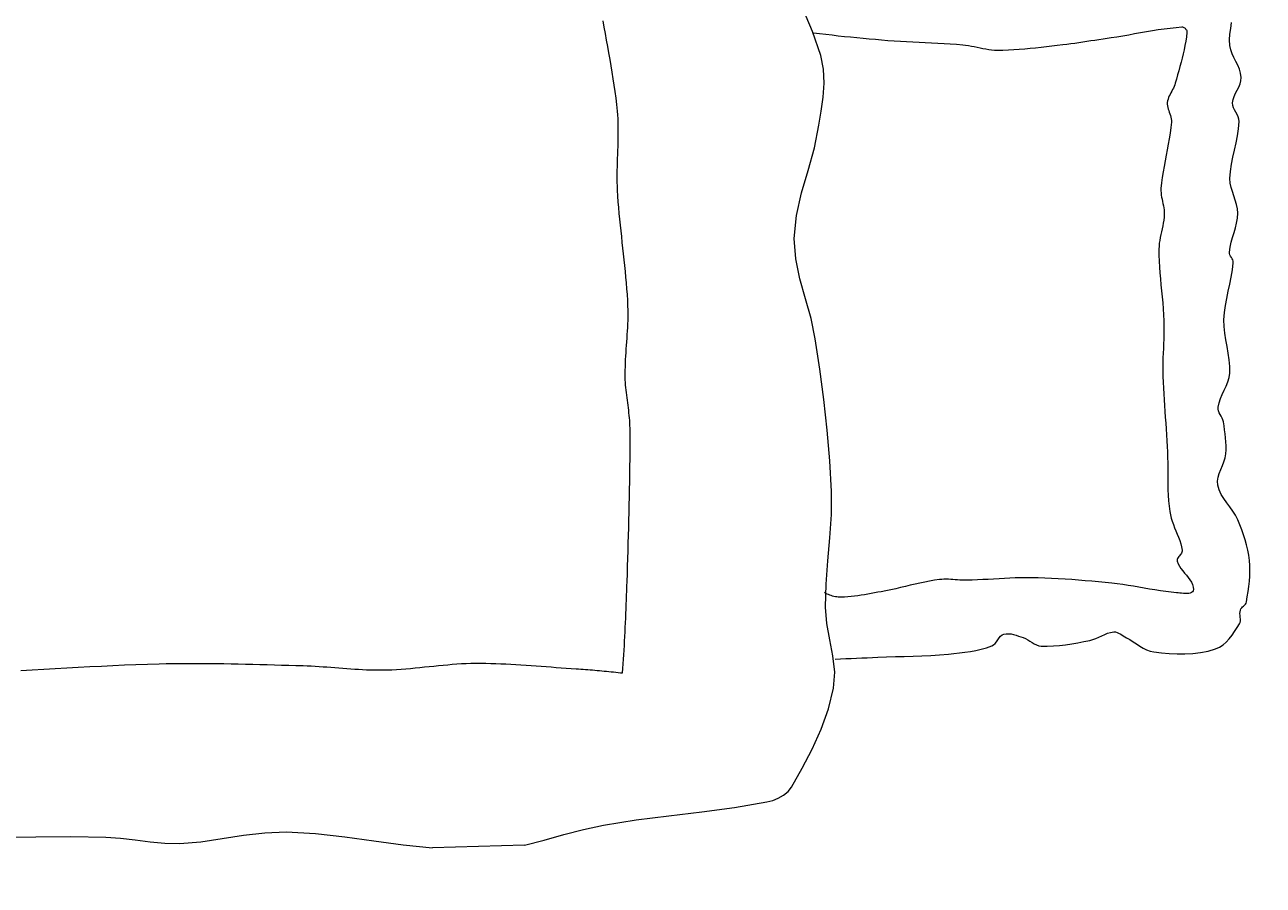
# Model space of a CAD drawing. Units: inches. Extents: x 1441 to 2460, y 1648 to 2683.
# Tile 5 of 35: x 1830 to 1880, y 1866 to 1901. Entities that reach past the tile are written whole.
import ezdxf

# ---------------------------------------------------------------- set-up
doc = ezdxf.new("R2010")
doc.units = ezdxf.units.IN
doc.layers.add('A-ANNO-DIMS', color=2, linetype='Continuous', lineweight=18)
doc.layers.add('A-FURN', color=8, linetype='Continuous', lineweight=15)
doc.styles.get("Standard").update_dxf_attribs({"font": 'arial.ttf'})
doc.dimstyles.get("Standard").update_dxf_attribs({"dimtxt": 0.18, "dimasz": 0.18, "dimexe": 0.18, "dimexo": 0.0625, "dimgap": 0.09, "dimtad": 0, "dimtih": 1, "dimtoh": 1, "dimdec": 4, "dimzin": 0, "dimdsep": 46, "dimtxsty": 'Standard', "dimcen": 0.09, "dimadec": 0, "dimazin": 0, "dimtfac": 1, "dimtdec": 4, "dimtofl": 0, "dimtmove": 0, "dimatfit": 3, "dimfxl": 1, "dimtolj": 1, "dimtzin": 0, "dimarcsym": 0})

# ---------------------------------------------------------------- blocks, each defined once
blk = doc.blocks.new('BED-DOUBLE-PLAN')
for p, q in [((52.61, 91.603), (52.404, 91.554)), ((52.818, 91.642), (52.61, 91.603)), ((53.027, 91.67), (52.818, 91.642)), ((53.234, 91.686), (53.027, 91.67)), ((53.441, 91.69), (53.234, 91.686)), ((53.649, 91.684), (53.441, 91.69)), ((53.857, 91.67), (53.649, 91.684)), ((54.065, 91.648), (53.857, 91.67)), ((54.272, 91.619), (54.065, 91.648)), ((54.478, 91.587), (54.272, 91.619)), ((54.683, 91.551), (54.478, 91.587)), ((33.099, 91.129), (32.945, 91.051)), ((33.253, 91.205), (33.099, 91.129)), ((33.41, 91.271), (33.253, 91.205)), ((33.569, 91.32), (33.41, 91.271)), ((33.735, 91.343), (33.569, 91.32)), ((33.867, 91.333), (33.735, 91.343)), ((33.995, 91.298), (33.867, 91.333)), ((34.121, 91.245), (33.995, 91.298)), ((34.245, 91.181), (34.121, 91.245)), ((34.37, 91.117), (34.245, 91.181)), ((34.495, 91.058), (34.37, 91.117)), ((35.036, 91.076), (34.945, 91.032)), ((35.126, 91.127), (35.036, 91.076)), ((35.216, 91.178), (35.126, 91.127)), ((35.307, 91.222), (35.216, 91.178)), ((35.4, 91.252), (35.307, 91.222)), ((35.496, 91.261), (35.4, 91.252)), ((35.784, 91.238), (35.496, 91.261)), ((36.07, 91.194), (35.784, 91.238)), ((36.354, 91.135), (36.07, 91.194)), ((36.638, 91.07), (36.354, 91.135)), ((36.922, 91.006), (36.638, 91.07)), ((38.639, 91.107), (38.469, 91.048)), ((38.81, 91.159), (38.639, 91.107)), ((38.983, 91.195), (38.81, 91.159)), ((39.158, 91.208), (38.983, 91.195)), ((39.356, 91.195), (39.158, 91.208)), ((39.551, 91.161), (39.356, 91.195)), ((39.744, 91.114), (39.551, 91.161)), ((39.936, 91.058), (39.744, 91.114)), ((51.224, 91.115), (51.053, 91.006)), ((51.403, 91.204), (51.224, 91.115)), ((51.599, 91.285), (51.403, 91.204)), ((51.797, 91.361), (51.599, 91.285)), ((51.997, 91.432), (51.797, 91.361)), ((52.2, 91.497), (51.997, 91.432)), ((52.404, 91.554), (52.2, 91.497)), ((54.729, 91.535), (54.683, 91.551)), ((54.771, 91.509), (54.729, 91.535)), ((54.81, 91.475), (54.771, 91.509)), ((54.847, 91.437), (54.81, 91.475)), ((54.884, 91.398), (54.847, 91.437)), ((54.922, 91.361), (54.884, 91.398)), ((54.963, 91.331), (54.922, 91.361)), ((55.008, 91.31), (54.963, 91.331)), ((55.076, 91.296), (55.008, 91.31)), ((55.147, 91.294), (55.076, 91.296)), ((55.219, 91.299), (55.147, 91.294)), ((55.292, 91.306), (55.219, 91.299)), ((55.364, 91.311), (55.292, 91.306)), ((55.433, 91.31), (55.364, 91.311)), ((55.499, 91.298), (55.433, 91.31)), ((55.56, 91.27), (55.499, 91.298)), ((55.709, 91.176), (55.56, 91.27)), ((55.86, 91.078), (55.709, 91.176)), ((56.01, 90.975), (55.86, 91.078)), ((31.78, 90.922), (31.549, 90.959)), ((32.011, 90.889), (31.78, 90.922)), ((32.24, 90.873), (32.011, 90.889)), ((32.466, 90.885), (32.24, 90.873)), ((32.63, 90.922), (32.466, 90.885)), ((32.789, 90.98), (32.63, 90.922)), ((32.945, 91.051), (32.789, 90.98)), ((34.624, 91.015), (34.495, 91.058)), ((34.756, 90.994), (34.624, 91.015)), ((34.852, 91.003), (34.756, 90.994)), ((34.945, 91.032), (34.852, 91.003)), ((37.206, 90.949), (36.922, 91.006)), ((37.492, 90.908), (37.206, 90.949)), ((37.78, 90.89), (37.492, 90.908)), ((37.955, 90.902), (37.78, 90.89)), ((38.128, 90.938), (37.955, 90.902)), ((38.299, 90.989), (38.128, 90.938)), ((38.469, 91.048), (38.299, 90.989)), ((40.129, 91), (39.936, 91.058)), ((40.322, 90.946), (40.129, 91)), ((40.516, 90.901), (40.322, 90.946)), ((40.713, 90.873), (40.516, 90.901)), ((40.767, 90.876), (40.713, 90.873)), ((40.821, 90.893), (40.767, 90.876)), ((40.873, 90.918), (40.821, 90.893)), ((40.924, 90.949), (40.873, 90.918)), ((40.975, 90.979), (40.924, 90.949)), ((41.027, 91.005), (40.975, 90.979)), ((41.081, 91.022), (41.027, 91.005)), ((41.135, 91.025), (41.081, 91.022)), ((41.423, 90.993), (41.135, 91.025)), ((41.708, 90.945), (41.423, 90.993)), ((41.993, 90.887), (41.708, 90.945)), ((42.277, 90.826), (41.993, 90.887)), ((42.561, 90.766), (42.277, 90.826)), ((42.845, 90.714), (42.561, 90.766)), ((43.131, 90.675), (42.845, 90.714)), ((43.419, 90.654), (43.131, 90.675)), ((43.686, 90.66), (43.419, 90.654)), ((43.952, 90.687), (43.686, 90.66)), ((44.218, 90.73), (43.952, 90.687)), ((44.483, 90.779), (44.218, 90.73)), ((44.748, 90.826), (44.483, 90.779)), ((45.014, 90.865), (44.748, 90.826)), ((45.28, 90.887), (45.014, 90.865)), ((45.546, 90.884), (45.28, 90.887)), ((45.723, 90.857), (45.546, 90.884)), ((45.894, 90.807), (45.723, 90.857)), ((46.062, 90.739), (45.894, 90.807)), ((46.228, 90.663), (46.062, 90.739)), ((46.394, 90.585), (46.228, 90.663)), ((46.562, 90.514), (46.394, 90.585)), ((47.342, 90.578), (47.27, 90.541)), ((47.415, 90.609), (47.342, 90.578)), ((47.49, 90.629), (47.415, 90.609)), ((47.648, 90.655), (47.49, 90.629)), ((47.807, 90.68), (47.648, 90.655)), ((47.967, 90.702), (47.807, 90.68)), ((48.127, 90.721), (47.967, 90.702)), ((48.287, 90.734), (48.127, 90.721)), ((48.447, 90.741), (48.287, 90.734)), ((48.607, 90.741), (48.447, 90.741)), ((48.767, 90.731), (48.607, 90.741)), ((48.926, 90.703), (48.767, 90.731)), ((49.084, 90.654), (48.926, 90.703)), ((49.24, 90.592), (49.084, 90.654)), ((49.395, 90.526), (49.24, 90.592)), ((50.558, 90.646), (50.387, 90.542)), ((50.723, 90.763), (50.558, 90.646)), ((50.888, 90.886), (50.723, 90.763)), ((51.053, 91.006), (50.888, 90.886)), ((56.153, 90.865), (56.01, 90.975)), ((56.284, 90.746), (56.153, 90.865)), ((56.399, 90.616), (56.284, 90.746)), ((56.493, 90.473), (56.399, 90.616)), ((46.733, 90.456), (46.562, 90.514)), ((46.908, 90.42), (46.733, 90.456)), ((46.984, 90.419), (46.908, 90.42)), ((47.057, 90.436), (46.984, 90.419)), ((47.128, 90.465), (47.057, 90.436)), ((47.199, 90.502), (47.128, 90.465)), ((47.27, 90.541), (47.199, 90.502)), ((49.549, 90.466), (49.395, 90.526)), ((49.704, 90.42), (49.549, 90.466)), ((49.861, 90.397), (49.704, 90.42)), ((50.019, 90.406), (49.861, 90.397)), ((50.209, 90.459), (50.019, 90.406)), ((50.387, 90.542), (50.209, 90.459)), ((56.561, 90.317), (56.493, 90.473)), ((56.643, 90.02), (56.561, 90.317)), ((56.701, 89.716), (56.643, 90.02)), ((56.736, 89.408), (56.701, 89.716)), ((31.755, 89.074), (31.774, 89.097)), ((31.774, 89.097), (31.795, 89.117)), ((31.795, 89.117), (31.818, 89.136)), ((31.818, 89.136), (31.843, 89.151)), ((31.843, 89.151), (31.869, 89.163)), ((31.869, 89.163), (31.896, 89.172)), ((31.896, 89.172), (31.922, 89.176)), ((31.922, 89.176), (31.948, 89.176)), ((31.948, 89.176), (32.119, 89.153)), ((32.119, 89.153), (32.29, 89.126)), ((32.29, 89.126), (32.459, 89.095)), ((32.459, 89.095), (32.629, 89.06)), ((53.527, 89.081), (53.616, 89.156)), ((53.616, 89.156), (53.705, 89.228)), ((53.705, 89.228), (53.796, 89.294)), ((53.796, 89.294), (53.889, 89.351)), ((53.889, 89.351), (53.985, 89.396)), ((53.985, 89.396), (54.086, 89.424)), ((54.086, 89.424), (54.192, 89.433)), ((54.192, 89.433), (54.243, 89.423)), ((54.243, 89.423), (54.282, 89.397)), ((54.282, 89.397), (54.31, 89.358)), ((54.31, 89.358), (54.329, 89.307)), ((54.329, 89.307), (54.341, 89.247)), ((54.341, 89.247), (54.346, 89.18)), ((54.346, 89.109), (54.342, 89.035)), ((54.346, 89.18), (54.346, 89.109)), ((56.752, 89.096), (56.736, 89.408)), ((56.751, 88.783), (56.752, 89.096)), ((31.722, 88.975), (31.723, 89)), ((31.741, 88.737), (31.722, 88.975)), ((31.723, 89), (31.729, 89.025)), ((31.729, 89.025), (31.74, 89.05)), ((31.74, 89.05), (31.755, 89.074)), ((31.765, 88.499), (31.741, 88.737)), ((32.629, 89.06), (32.797, 89.023)), ((32.797, 89.023), (32.966, 88.982)), ((32.966, 88.982), (33.133, 88.94)), ((33.133, 88.94), (33.301, 88.895)), ((33.301, 88.895), (33.468, 88.85)), ((33.468, 88.85), (33.635, 88.803)), ((33.635, 88.803), (33.801, 88.756)), ((33.801, 88.756), (33.968, 88.709)), ((33.968, 88.709), (34.034, 88.688)), ((34.034, 88.688), (34.099, 88.662)), ((34.099, 88.662), (34.162, 88.632)), ((34.162, 88.632), (34.225, 88.599)), ((34.225, 88.599), (34.288, 88.566)), ((51.463, 88.586), (51.591, 88.632)), ((51.591, 88.632), (51.719, 88.683)), ((51.719, 88.683), (51.846, 88.735)), ((51.846, 88.735), (51.972, 88.787)), ((51.972, 88.787), (52.1, 88.838)), ((52.1, 88.838), (52.228, 88.885)), ((52.228, 88.885), (52.357, 88.926)), ((52.357, 88.926), (52.488, 88.961)), ((52.488, 88.961), (52.621, 88.986)), ((52.621, 88.986), (52.66, 88.986)), ((52.66, 88.986), (52.697, 88.976)), ((52.697, 88.976), (52.734, 88.958)), ((52.734, 88.958), (52.769, 88.934)), ((52.769, 88.934), (52.804, 88.906)), ((52.804, 88.906), (52.839, 88.877)), ((52.839, 88.877), (52.873, 88.848)), ((52.873, 88.848), (52.908, 88.822)), ((52.908, 88.822), (52.943, 88.8)), ((52.943, 88.8), (52.979, 88.785)), ((52.979, 88.785), (53.015, 88.778)), ((53.015, 88.778), (53.053, 88.783)), ((53.053, 88.783), (53.155, 88.821)), ((53.155, 88.821), (53.253, 88.873)), ((53.253, 88.873), (53.347, 88.936)), ((53.347, 88.936), (53.438, 89.006)), ((53.438, 89.006), (53.527, 89.081)), ((54.315, 88.761), (54.295, 88.544)), ((54.321, 88.821), (54.315, 88.761)), ((54.328, 88.889), (54.321, 88.821)), ((54.335, 88.961), (54.328, 88.889)), ((54.342, 89.035), (54.335, 88.961)), ((56.736, 88.47), (56.751, 88.783)), ((31.795, 88.263), (31.765, 88.499)), ((31.829, 88.027), (31.795, 88.263)), ((34.288, 88.566), (34.35, 88.532)), ((34.35, 88.532), (34.413, 88.5)), ((34.413, 88.5), (34.476, 88.469)), ((34.476, 88.469), (34.54, 88.442)), ((34.54, 88.442), (34.605, 88.419)), ((34.605, 88.419), (34.671, 88.401)), ((34.671, 88.401), (34.739, 88.39)), ((34.739, 88.39), (34.805, 88.388)), ((34.805, 88.388), (34.87, 88.394)), ((34.87, 88.394), (34.935, 88.407)), ((34.935, 88.407), (35, 88.425)), ((35, 88.425), (35.064, 88.446)), ((35.064, 88.446), (35.128, 88.468)), ((35.128, 88.468), (35.193, 88.491)), ((35.193, 88.491), (35.257, 88.513)), ((35.257, 88.513), (35.322, 88.531)), ((35.322, 88.531), (35.387, 88.545)), ((35.387, 88.545), (35.452, 88.552)), ((35.452, 88.552), (35.518, 88.552)), ((35.518, 88.552), (35.741, 88.531)), ((35.741, 88.531), (35.963, 88.503)), ((35.963, 88.503), (36.184, 88.469)), ((36.184, 88.469), (36.405, 88.43)), ((36.405, 88.43), (36.626, 88.388)), ((36.626, 88.388), (36.847, 88.345)), ((36.847, 88.345), (37.067, 88.302)), ((37.067, 88.302), (37.288, 88.26)), ((37.288, 88.26), (37.509, 88.221)), ((37.509, 88.221), (37.73, 88.187)), ((37.73, 88.187), (37.953, 88.158)), ((37.953, 88.158), (38.176, 88.137)), ((38.176, 88.137), (38.262, 88.134)), ((38.262, 88.134), (38.347, 88.138)), ((38.347, 88.138), (38.433, 88.148)), ((38.433, 88.148), (38.518, 88.162)), ((38.518, 88.162), (38.604, 88.178)), ((38.604, 88.178), (38.689, 88.197)), ((38.689, 88.197), (38.774, 88.216)), ((38.774, 88.216), (38.86, 88.233)), ((38.86, 88.233), (38.945, 88.249)), ((38.945, 88.249), (39.031, 88.261)), ((39.031, 88.261), (39.117, 88.268)), ((39.117, 88.268), (39.203, 88.268)), ((39.203, 88.268), (39.32, 88.261)), ((39.32, 88.261), (39.437, 88.247)), ((39.437, 88.247), (39.553, 88.228)), ((39.553, 88.228), (39.668, 88.206)), ((39.668, 88.206), (39.783, 88.181)), ((39.783, 88.181), (39.899, 88.155)), ((39.899, 88.155), (40.014, 88.13)), ((40.014, 88.13), (40.13, 88.106)), ((40.13, 88.106), (40.245, 88.085)), ((41.547, 88.095), (41.785, 88.115)), ((41.785, 88.115), (42.023, 88.137)), ((42.023, 88.137), (42.261, 88.16)), ((42.261, 88.16), (42.499, 88.183)), ((42.499, 88.183), (42.737, 88.204)), ((42.737, 88.204), (42.975, 88.222)), ((42.975, 88.222), (43.213, 88.237)), ((43.213, 88.237), (43.451, 88.247)), ((43.451, 88.247), (43.636, 88.251)), ((43.636, 88.251), (43.822, 88.251)), ((43.822, 88.251), (44.007, 88.249)), ((44.007, 88.249), (44.192, 88.244)), ((44.192, 88.244), (44.377, 88.238)), ((44.377, 88.238), (44.562, 88.231)), ((44.562, 88.231), (44.748, 88.224)), ((44.748, 88.224), (44.933, 88.217)), ((44.933, 88.217), (45.118, 88.212)), ((45.118, 88.212), (45.303, 88.209)), ((45.303, 88.209), (45.488, 88.209)), ((45.488, 88.209), (45.674, 88.212)), ((45.674, 88.212), (45.907, 88.22)), ((45.907, 88.22), (46.141, 88.231)), ((46.141, 88.231), (46.375, 88.244)), ((46.375, 88.244), (46.609, 88.259)), ((46.609, 88.259), (46.842, 88.275)), ((46.842, 88.275), (47.076, 88.292)), ((47.076, 88.292), (47.309, 88.309)), ((47.309, 88.309), (47.543, 88.327)), ((47.543, 88.327), (47.776, 88.344)), ((47.776, 88.344), (48.01, 88.36)), ((48.01, 88.36), (48.243, 88.374)), ((48.243, 88.374), (48.477, 88.387)), ((48.477, 88.387), (48.693, 88.396)), ((48.693, 88.396), (48.91, 88.401)), ((48.91, 88.401), (49.126, 88.404)), ((49.126, 88.404), (49.343, 88.405)), ((49.343, 88.405), (49.56, 88.406)), ((49.56, 88.406), (49.776, 88.407)), ((49.776, 88.407), (49.993, 88.41)), ((49.993, 88.41), (50.209, 88.415)), ((50.209, 88.415), (50.425, 88.425)), ((50.425, 88.425), (50.64, 88.439)), ((50.64, 88.439), (50.855, 88.459)), ((50.855, 88.459), (51.07, 88.486)), ((51.07, 88.486), (51.203, 88.511)), ((51.203, 88.511), (51.334, 88.544)), ((51.334, 88.544), (51.463, 88.586)), ((54.239, 88.112), (54.205, 87.897)), ((54.269, 88.328), (54.239, 88.112)), ((54.295, 88.544), (54.269, 88.328)), ((56.674, 87.849), (56.709, 88.158)), ((56.709, 88.158), (56.736, 88.47)), ((31.866, 87.791), (31.829, 88.027)), ((31.905, 87.555), (31.866, 87.791)), ((40.245, 88.085), (40.361, 88.069)), ((40.361, 88.069), (40.478, 88.058)), ((40.478, 88.058), (40.595, 88.053)), ((40.595, 88.053), (40.833, 88.055)), ((40.833, 88.055), (41.071, 88.064)), ((41.071, 88.064), (41.309, 88.077)), ((41.309, 88.077), (41.547, 88.095)), ((54.169, 87.682), (54.132, 87.467)), ((54.205, 87.897), (54.169, 87.682)), ((56.591, 87.558), (56.643, 87.7)), ((56.643, 87.7), (56.674, 87.849)), ((31.946, 87.319), (31.905, 87.555)), ((31.988, 87.084), (31.946, 87.319)), ((54.094, 87.252), (54.057, 87.037)), ((54.132, 87.467), (54.094, 87.252)), ((56.272, 87.021), (56.359, 87.153)), ((56.359, 87.153), (56.444, 87.286)), ((56.444, 87.286), (56.523, 87.42)), ((56.523, 87.42), (56.591, 87.558)), ((32.03, 86.849), (31.988, 87.084)), ((32.071, 86.613), (32.03, 86.849)), ((32.11, 86.377), (32.071, 86.613)), ((54.021, 86.822), (53.988, 86.607)), ((54.057, 87.037), (54.021, 86.822)), ((56, 86.568), (56.041, 86.629)), ((56.041, 86.629), (56.08, 86.69)), ((56.08, 86.69), (56.114, 86.752)), ((56.114, 86.752), (56.189, 86.888)), ((56.189, 86.888), (56.272, 87.021)), ((32.146, 86.141), (32.11, 86.377)), ((32.17, 85.981), (32.146, 86.141)), ((53.934, 86.174), (53.907, 85.907)), ((53.959, 86.391), (53.934, 86.174)), ((53.988, 86.607), (53.959, 86.391)), ((55.878, 86.248), (55.881, 86.316)), ((55.897, 86.124), (55.878, 86.248)), ((55.881, 86.316), (55.898, 86.382)), ((55.933, 86.004), (55.897, 86.124)), ((55.898, 86.382), (55.925, 86.445)), ((55.925, 86.445), (55.96, 86.507)), ((55.96, 86.507), (56, 86.568)), ((32.195, 85.82), (32.17, 85.981)), ((32.22, 85.659), (32.195, 85.82)), ((32.245, 85.499), (32.22, 85.659)), ((53.881, 85.64), (53.857, 85.373)), ((53.907, 85.907), (53.881, 85.64)), ((55.98, 85.887), (55.933, 86.004)), ((56.034, 85.771), (55.98, 85.887)), ((56.09, 85.655), (56.034, 85.771)), ((56.144, 85.538), (56.09, 85.655)), ((32.269, 85.338), (32.245, 85.499)), ((32.294, 85.177), (32.269, 85.338)), ((32.318, 85.017), (32.294, 85.177)), ((53.857, 85.373), (53.834, 85.105)), ((56.189, 85.419), (56.144, 85.538)), ((56.221, 85.297), (56.189, 85.419)), ((56.268, 85.056), (56.221, 85.297)), ((32.342, 84.856), (32.318, 85.017)), ((32.364, 84.695), (32.342, 84.856)), ((32.385, 84.534), (32.364, 84.695)), ((53.813, 84.838), (53.793, 84.57)), ((53.834, 85.105), (53.813, 84.838)), ((56.313, 84.813), (56.268, 85.056)), ((56.355, 84.57), (56.313, 84.813)), ((32.406, 84.372), (32.385, 84.534)), ((32.424, 84.211), (32.406, 84.372)), ((32.449, 83.994), (32.424, 84.211)), ((53.775, 84.302), (53.76, 84.034)), ((53.793, 84.57), (53.775, 84.302)), ((56.391, 84.327), (56.355, 84.57)), ((56.42, 84.082), (56.391, 84.327)), ((32.474, 83.778), (32.449, 83.994)), ((32.499, 83.561), (32.474, 83.778)), ((53.746, 83.766), (53.735, 83.498)), ((53.76, 84.034), (53.746, 83.766)), ((56.44, 83.838), (56.42, 84.082)), ((56.45, 83.593), (56.44, 83.838)), ((32.524, 83.344), (32.499, 83.561)), ((32.549, 83.127), (32.524, 83.344)), ((53.725, 83.23), (53.719, 82.961)), ((53.735, 83.498), (53.725, 83.23)), ((56.356, 83.07), (56.4, 83.159)), ((56.4, 83.159), (56.432, 83.251)), ((56.432, 83.251), (56.446, 83.348)), ((56.446, 83.348), (56.45, 83.593)), ((32.571, 82.909), (32.549, 83.127)), ((32.592, 82.692), (32.571, 82.909)), ((32.61, 82.475), (32.592, 82.692)), ((53.719, 82.961), (53.717, 82.745)), ((53.717, 82.745), (53.719, 82.529)), ((56.108, 82.628), (56.146, 82.721)), ((56.146, 82.721), (56.194, 82.81)), ((56.194, 82.81), (56.248, 82.897)), ((56.248, 82.897), (56.304, 82.983)), ((56.304, 82.983), (56.356, 83.07)), ((32.625, 82.257), (32.61, 82.475)), ((32.637, 82.04), (32.625, 82.257)), ((53.719, 82.529), (53.725, 82.313)), ((53.725, 82.313), (53.733, 82.097)), ((55.961, 82.149), (55.983, 82.246)), ((55.983, 82.246), (56.011, 82.343)), ((56.011, 82.343), (56.043, 82.439)), ((56.043, 82.439), (56.077, 82.535)), ((56.077, 82.535), (56.108, 82.628)), ((32.645, 81.822), (32.637, 82.04)), ((32.648, 81.604), (32.645, 81.822)), ((53.733, 82.097), (53.743, 81.881)), ((53.743, 81.881), (53.755, 81.665)), ((53.755, 81.665), (53.768, 81.449)), ((55.95, 82.052), (55.961, 82.149)), ((55.951, 81.956), (55.95, 82.052)), ((55.967, 81.861), (55.951, 81.956)), ((56.001, 81.786), (55.967, 81.861)), ((56.055, 81.723), (56.001, 81.786)), ((56.122, 81.667), (56.055, 81.723)), ((56.197, 81.616), (56.122, 81.667)), ((32.602, 81.139), (32.62, 81.254)), ((32.62, 81.254), (32.635, 81.37)), ((32.635, 81.37), (32.644, 81.487)), ((32.644, 81.487), (32.648, 81.604)), ((53.768, 81.449), (53.78, 81.233)), ((53.78, 81.233), (53.792, 81.017)), ((56.273, 81.564), (56.197, 81.616)), ((56.343, 81.51), (56.273, 81.564)), ((56.401, 81.448), (56.343, 81.51)), ((56.441, 81.375), (56.401, 81.448)), ((56.51, 81.165), (56.441, 81.375)), ((32.484, 80.561), (32.507, 80.677)), ((32.507, 80.677), (32.532, 80.792)), ((32.532, 80.792), (32.556, 80.908)), ((32.556, 80.908), (32.58, 81.023)), ((32.58, 81.023), (32.602, 81.139)), ((53.792, 81.017), (53.803, 80.801)), ((53.803, 80.801), (53.812, 80.585)), ((56.568, 80.953), (56.51, 81.165)), ((56.617, 80.737), (56.568, 80.953)), ((56.657, 80.52), (56.617, 80.737)), ((32.412, 79.964), (32.433, 80.213)), ((32.433, 80.213), (32.446, 80.329)), ((32.446, 80.329), (32.463, 80.445)), ((32.463, 80.445), (32.484, 80.561)), ((53.815, 80.188), (53.81, 80.097)), ((53.812, 80.585), (53.817, 80.369)), ((53.817, 80.278), (53.815, 80.188)), ((53.817, 80.369), (53.817, 80.278)), ((56.691, 80.301), (56.657, 80.52)), ((56.72, 80.081), (56.691, 80.301)), ((32.379, 79.466), (32.394, 79.715)), ((32.394, 79.715), (32.412, 79.964)), ((53.782, 79.735), (53.778, 79.644)), ((53.789, 79.825), (53.782, 79.735)), ((53.796, 79.916), (53.789, 79.825)), ((53.803, 80.007), (53.796, 79.916)), ((53.81, 80.097), (53.803, 80.007)), ((56.745, 79.861), (56.72, 80.081)), ((56.767, 79.641), (56.745, 79.861)), ((32.353, 78.967), (32.365, 79.217)), ((32.365, 79.217), (32.379, 79.466)), ((53.778, 79.644), (53.776, 79.554)), ((53.776, 79.554), (53.776, 79.464)), ((53.776, 79.464), (53.781, 79.374)), ((53.781, 79.374), (53.791, 79.284)), ((53.791, 79.284), (53.819, 79.088)), ((56.798, 79.289), (56.767, 79.641)), ((56.82, 78.937), (56.798, 79.289)), ((32.33, 78.469), (32.341, 78.718)), ((32.341, 78.718), (32.353, 78.967)), ((53.819, 79.088), (53.853, 78.892)), ((53.853, 78.892), (53.891, 78.697)), ((53.891, 78.697), (53.932, 78.503)), ((56.836, 78.584), (56.82, 78.937)), ((32.305, 77.97), (32.318, 78.219)), ((32.318, 78.219), (32.33, 78.469)), ((53.932, 78.503), (53.975, 78.309)), ((53.975, 78.309), (54.019, 78.115)), ((56.848, 78.231), (56.836, 78.584)), ((56.857, 77.878), (56.848, 78.231)), ((32.275, 77.472), (32.291, 77.721)), ((32.291, 77.721), (32.305, 77.97)), ((54.019, 78.115), (54.065, 77.922)), ((54.065, 77.922), (54.11, 77.728)), ((54.11, 77.728), (54.154, 77.534)), ((56.866, 77.524), (56.857, 77.878)), ((32.237, 76.974), (32.257, 77.223)), ((32.257, 77.223), (32.275, 77.472)), ((54.154, 77.534), (54.197, 77.34)), ((54.197, 77.34), (54.237, 77.145)), ((56.876, 77.171), (56.866, 77.524)), ((32.193, 76.478), (32.215, 76.726)), ((32.215, 76.726), (32.237, 76.974)), ((54.237, 77.145), (54.274, 76.95)), ((54.274, 76.95), (54.298, 76.818)), ((54.298, 76.818), (54.322, 76.686)), ((56.89, 76.818), (56.876, 77.171)), ((56.899, 76.605), (56.89, 76.818)), ((32.147, 75.981), (32.17, 76.23)), ((32.17, 76.23), (32.193, 76.478)), ((54.322, 76.686), (54.346, 76.554)), ((54.346, 76.554), (54.37, 76.421)), ((54.37, 76.421), (54.393, 76.289)), ((54.393, 76.289), (54.414, 76.156)), ((56.908, 76.392), (56.899, 76.605)), ((56.918, 76.179), (56.908, 76.392)), ((32.097, 75.486), (32.122, 75.733)), ((32.122, 75.733), (32.147, 75.981)), ((54.414, 76.156), (54.434, 76.023)), ((54.434, 76.023), (54.451, 75.89)), ((54.451, 75.89), (54.466, 75.757)), ((54.466, 75.757), (54.478, 75.624)), ((56.928, 75.966), (56.918, 76.179)), ((56.937, 75.753), (56.928, 75.966)), ((56.947, 75.54), (56.937, 75.753)), ((32.043, 74.99), (32.07, 75.238)), ((32.07, 75.238), (32.097, 75.486)), ((54.478, 75.624), (54.486, 75.49)), ((54.487, 75.241), (54.481, 75.184)), ((54.486, 75.49), (54.49, 75.356)), ((54.49, 75.299), (54.487, 75.241)), ((54.49, 75.356), (54.49, 75.299)), ((56.957, 75.327), (56.947, 75.54)), ((56.967, 75.114), (56.957, 75.327)), ((31.986, 74.495), (32.015, 74.742)), ((32.015, 74.742), (32.043, 74.99)), ((47.824, 74.794), (46.604, 74.657)), ((49.046, 74.901), (47.824, 74.794)), ((50.27, 74.969), (49.046, 74.901)), ((51.196, 74.964), (50.27, 74.969)), ((52.121, 74.904), (51.196, 74.964)), ((53.045, 74.821), (52.121, 74.904)), ((53.971, 74.75), (53.045, 74.821)), ((54.897, 74.726), (53.971, 74.75)), ((54.34, 74.744), (54.311, 74.694)), ((54.366, 74.795), (54.34, 74.744)), ((54.39, 74.848), (54.366, 74.795)), ((54.411, 74.902), (54.39, 74.848)), ((54.43, 74.957), (54.411, 74.902)), ((54.447, 75.012), (54.43, 74.957)), ((54.461, 75.069), (54.447, 75.012)), ((54.472, 75.126), (54.461, 75.069)), ((54.481, 75.184), (54.472, 75.126)), ((55.545, 74.784), (54.897, 74.726)), ((56.194, 74.904), (55.545, 74.784)), ((56.84, 75.028), (56.194, 74.904)), ((57.484, 75.097), (56.84, 75.028)), ((58.123, 75.053), (57.484, 75.097)), ((58.956, 74.846), (58.123, 75.053)), ((59.766, 74.555), (58.956, 74.846)), ((32.864, 74.545), (31.901, 74.215)), ((31.956, 74.247), (31.986, 74.495)), ((33.405, 74.651), (32.864, 74.545)), ((33.96, 74.67), (33.405, 74.651)), ((34.522, 74.63), (33.96, 74.67)), ((35.083, 74.555), (34.522, 74.63)), ((35.638, 74.47), (35.083, 74.555)), ((36.55, 74.284), (35.638, 74.47)), ((37.452, 74.033), (36.55, 74.284)), ((44.172, 74.323), (43.37, 74.156)), ((45.387, 74.497), (44.172, 74.323)), ((46.604, 74.657), (45.387, 74.497)), ((60.555, 74.2), (59.766, 74.555)), ((31.901, 74.215), (30.964, 73.813)), ((38.351, 73.775), (37.452, 74.033)), ((39.257, 73.571), (38.351, 73.775)), ((42.576, 73.933), (41.783, 73.709)), ((43.37, 74.156), (42.576, 73.933)), ((61.324, 73.8), (60.555, 74.2)), ((62.074, 73.372), (61.324, 73.8)), ((40.176, 73.479), (39.257, 73.571)), ((40.985, 73.539), (40.176, 73.479)), ((41.783, 73.709), (40.985, 73.539)), ((62.255, 73.232), (62.074, 73.372)), ((62.403, 73.052), (62.255, 73.232)), ((62.52, 72.843), (62.403, 73.052)), ((62.608, 72.619), (62.52, 72.843)), ((62.667, 72.392), (62.608, 72.619)), ((62.893, 71.092), (62.667, 72.392)), ((63.068, 69.783), (62.893, 71.092)), ((63.223, 68.471), (63.068, 69.783)), ((63.387, 67.161), (63.223, 68.471)), ((42.639, 66.825), (42.407, 66.811)), ((42.871, 66.836), (42.639, 66.825)), ((43.013, 66.84), (42.871, 66.836)), ((43.155, 66.842), (43.013, 66.84)), ((43.298, 66.841), (43.155, 66.842)), ((43.44, 66.838), (43.298, 66.841)), ((43.582, 66.833), (43.44, 66.838)), ((43.724, 66.826), (43.582, 66.833)), ((43.867, 66.819), (43.724, 66.826)), ((44.009, 66.81), (43.867, 66.819)), ((46.727, 66.825), (46.627, 66.811)), ((46.828, 66.839), (46.727, 66.825)), ((46.929, 66.852), (46.828, 66.839)), ((47.03, 66.865), (46.929, 66.852)), ((47.131, 66.877), (47.03, 66.865)), ((47.232, 66.888), (47.131, 66.877)), ((47.333, 66.898), (47.232, 66.888)), ((47.434, 66.906), (47.333, 66.898)), ((47.535, 66.912), (47.434, 66.906)), ((47.637, 66.917), (47.535, 66.912)), ((47.738, 66.919), (47.637, 66.917)), ((48.045, 66.921), (47.738, 66.919)), ((48.352, 66.922), (48.045, 66.921)), ((48.658, 66.921), (48.352, 66.922)), ((48.965, 66.92), (48.658, 66.921)), ((49.272, 66.917), (48.965, 66.92)), ((49.579, 66.913), (49.272, 66.917)), ((49.885, 66.909), (49.579, 66.913)), ((50.192, 66.903), (49.885, 66.909)), ((50.499, 66.897), (50.192, 66.903)), ((50.806, 66.89), (50.499, 66.897)), ((51.112, 66.883), (50.806, 66.89)), ((51.419, 66.875), (51.112, 66.883)), ((51.726, 66.866), (51.419, 66.875)), ((52.032, 66.857), (51.726, 66.866)), ((52.339, 66.848), (52.032, 66.857)), ((52.646, 66.839), (52.339, 66.848)), ((52.952, 66.83), (52.646, 66.839)), ((53.259, 66.82), (52.952, 66.83)), ((53.566, 66.811), (53.259, 66.82)), ((63.59, 65.856), (63.387, 67.161)), ((34.303, 66.324), (34.045, 66.287)), ((34.561, 66.358), (34.303, 66.324)), ((34.82, 66.388), (34.561, 66.358)), ((35.079, 66.415), (34.82, 66.388)), ((35.237, 66.428), (35.079, 66.415)), ((35.394, 66.438), (35.237, 66.428)), ((35.552, 66.444), (35.394, 66.438)), ((35.71, 66.448), (35.552, 66.444)), ((35.868, 66.45), (35.71, 66.448)), ((36.026, 66.449), (35.868, 66.45)), ((36.184, 66.447), (36.026, 66.449)), ((36.343, 66.444), (36.184, 66.447)), ((36.501, 66.439), (36.343, 66.444)), ((36.66, 66.434), (36.501, 66.439)), ((36.818, 66.428), (36.66, 66.434)), ((36.976, 66.423), (36.818, 66.428)), ((37.135, 66.418), (36.976, 66.423)), ((37.293, 66.413), (37.135, 66.418)), ((37.451, 66.41), (37.293, 66.413)), ((37.61, 66.408), (37.451, 66.41)), ((37.768, 66.408), (37.61, 66.408)), ((37.926, 66.41), (37.768, 66.408)), ((38.084, 66.414), (37.926, 66.41)), ((38.242, 66.421), (38.084, 66.414)), ((38.474, 66.435), (38.242, 66.421)), ((38.706, 66.451), (38.474, 66.435)), ((38.938, 66.47), (38.706, 66.451)), ((39.169, 66.49), (38.938, 66.47)), ((39.4, 66.512), (39.169, 66.49)), ((39.632, 66.535), (39.4, 66.512)), ((39.863, 66.56), (39.632, 66.535)), ((40.094, 66.585), (39.863, 66.56)), ((40.325, 66.61), (40.094, 66.585)), ((40.556, 66.636), (40.325, 66.61)), ((40.787, 66.661), (40.556, 66.636)), ((41.018, 66.686), (40.787, 66.661)), ((41.25, 66.711), (41.018, 66.686)), ((41.481, 66.734), (41.25, 66.711)), ((41.712, 66.756), (41.481, 66.734)), ((41.944, 66.776), (41.712, 66.756)), ((42.175, 66.795), (41.944, 66.776)), ((42.407, 66.811), (42.175, 66.795)), ((44.151, 66.8), (44.009, 66.81)), ((44.294, 66.79), (44.151, 66.8)), ((44.436, 66.78), (44.294, 66.79)), ((44.578, 66.77), (44.436, 66.78)), ((44.72, 66.76), (44.578, 66.77)), ((44.863, 66.751), (44.72, 66.76)), ((45.005, 66.743), (44.863, 66.751)), ((45.147, 66.736), (45.005, 66.743)), ((45.29, 66.731), (45.147, 66.736)), ((45.432, 66.727), (45.29, 66.731)), ((45.574, 66.726), (45.432, 66.727)), ((45.717, 66.727), (45.574, 66.726)), ((45.818, 66.73), (45.717, 66.727)), ((45.92, 66.735), (45.818, 66.73)), ((46.021, 66.742), (45.92, 66.735)), ((46.122, 66.751), (46.021, 66.742)), ((46.223, 66.761), (46.122, 66.751)), ((46.324, 66.773), (46.223, 66.761)), ((46.425, 66.785), (46.324, 66.773)), ((46.526, 66.798), (46.425, 66.785)), ((46.627, 66.811), (46.526, 66.798)), ((53.872, 66.801), (53.566, 66.811)), ((54.055, 66.796), (53.872, 66.801)), ((54.237, 66.79), (54.055, 66.796)), ((54.42, 66.783), (54.237, 66.79)), ((54.602, 66.777), (54.42, 66.783)), ((54.785, 66.77), (54.602, 66.777)), ((54.967, 66.762), (54.785, 66.77)), ((55.15, 66.755), (54.967, 66.762)), ((55.332, 66.747), (55.15, 66.755)), ((55.515, 66.738), (55.332, 66.747)), ((55.697, 66.729), (55.515, 66.738)), ((55.879, 66.72), (55.697, 66.729)), ((56.062, 66.711), (55.879, 66.72)), ((56.244, 66.701), (56.062, 66.711)), ((56.426, 66.691), (56.244, 66.701)), ((56.609, 66.681), (56.426, 66.691)), ((56.791, 66.67), (56.609, 66.681)), ((56.973, 66.659), (56.791, 66.67)), ((57.155, 66.648), (56.973, 66.659)), ((57.338, 66.636), (57.155, 66.648)), ((57.52, 66.624), (57.338, 66.636)), ((57.479, 66.254), (57.489, 66.346)), ((57.489, 66.346), (57.499, 66.439)), ((57.499, 66.439), (57.509, 66.531)), ((57.509, 66.531), (57.52, 66.624)), ((31.732, 65.891), (31.475, 65.847)), ((31.989, 65.936), (31.732, 65.891)), ((32.246, 65.982), (31.989, 65.936)), ((32.502, 66.028), (32.246, 65.982)), ((32.759, 66.074), (32.502, 66.028)), ((33.016, 66.119), (32.759, 66.074)), ((33.273, 66.163), (33.016, 66.119)), ((33.53, 66.207), (33.273, 66.163)), ((33.787, 66.248), (33.53, 66.207)), ((34.045, 66.287), (33.787, 66.248)), ((57.433, 65.791), (57.442, 65.884)), ((57.442, 65.884), (57.451, 65.976)), ((57.451, 65.976), (57.46, 66.069)), ((57.46, 66.069), (57.469, 66.161)), ((57.469, 66.161), (57.479, 66.254)), ((63.763, 65.061), (63.59, 65.856)), ((57.393, 65.328), (57.4, 65.421)), ((57.4, 65.421), (57.408, 65.513)), ((57.408, 65.513), (57.416, 65.606)), ((57.416, 65.606), (57.425, 65.699)), ((57.425, 65.699), (57.433, 65.791)), ((57.352, 64.771), (57.358, 64.864)), ((57.358, 64.864), (57.364, 64.957)), ((57.364, 64.957), (57.371, 65.05)), ((57.371, 65.05), (57.378, 65.142)), ((57.378, 65.142), (57.385, 65.235)), ((57.385, 65.235), (57.393, 65.328)), ((63.975, 64.273), (63.763, 65.061)), ((57.309, 64.168), (57.324, 64.369)), ((57.324, 64.369), (57.338, 64.57)), ((57.338, 64.57), (57.352, 64.771)), ((57.278, 63.767), (57.294, 63.968)), ((57.294, 63.968), (57.309, 64.168)), ((64.196, 63.488), (63.975, 64.273)), ((57.233, 63.164), (57.248, 63.365)), ((57.248, 63.365), (57.263, 63.566)), ((57.263, 63.566), (57.278, 63.767)), ((64.395, 62.698), (64.196, 63.488)), ((57.204, 62.762), (57.218, 62.963)), ((57.218, 62.963), (57.233, 63.164)), ((57.179, 62.359), (57.191, 62.56)), ((57.191, 62.56), (57.204, 62.762)), ((64.395, 62.698), (64.503, 59.019)), ((57.149, 61.756), (57.157, 61.957)), ((57.157, 61.957), (57.168, 62.158)), ((57.168, 62.158), (57.179, 62.359)), ((57.136, 61.353), (57.141, 61.555)), ((57.141, 61.555), (57.149, 61.756)), ((57.13, 60.951), (57.132, 61.152)), ((57.13, 60.749), (57.13, 60.951)), ((57.132, 61.152), (57.136, 61.353)), ((57.133, 60.563), (57.13, 60.749)), ((57.139, 60.376), (57.133, 60.563)), ((57.147, 60.19), (57.139, 60.376)), ((57.159, 60.003), (57.147, 60.19)), ((57.172, 59.817), (57.159, 60.003)), ((57.188, 59.631), (57.172, 59.817)), ((57.205, 59.445), (57.188, 59.631)), ((57.222, 59.259), (57.205, 59.445)), ((57.241, 59.073), (57.222, 59.259)), ((57.26, 58.887), (57.241, 59.073)), ((64.382, 57.848), (64.503, 59.019)), ((57.279, 58.701), (57.26, 58.887)), ((57.298, 58.515), (57.279, 58.701)), ((57.317, 58.328), (57.298, 58.515)), ((57.334, 58.142), (57.317, 58.328)), ((57.35, 57.956), (57.334, 58.142)), ((57.364, 57.77), (57.35, 57.956)), ((57.377, 57.584), (57.364, 57.77)), ((57.387, 57.397), (57.377, 57.584)), ((64.222, 56.681), (64.382, 57.848)), ((57.394, 57.211), (57.387, 57.397)), ((57.398, 57.024), (57.394, 57.211)), ((57.399, 56.865), (57.398, 57.024)), ((57.389, 56.39), (57.394, 56.548)), ((57.394, 56.548), (57.398, 56.707)), ((57.398, 56.707), (57.399, 56.865)), ((64.06, 55.515), (64.222, 56.681)), ((57.363, 55.915), (57.373, 56.073)), ((57.373, 56.073), (57.382, 56.232)), ((57.382, 56.232), (57.389, 56.39)), ((57.316, 55.282), (57.329, 55.44)), ((57.329, 55.44), (57.341, 55.598)), ((57.341, 55.598), (57.353, 55.757)), ((57.353, 55.757), (57.363, 55.915)), ((63.929, 54.347), (64.06, 55.515)), ((57.279, 54.807), (57.291, 54.965)), ((57.291, 54.965), (57.304, 55.123)), ((57.304, 55.123), (57.316, 55.282)), ((57.247, 54.332), (57.257, 54.49)), ((57.257, 54.49), (57.268, 54.649)), ((57.268, 54.649), (57.279, 54.807)), ((57.227, 53.856), (57.232, 54.015)), ((57.232, 54.015), (57.239, 54.173)), ((57.239, 54.173), (57.247, 54.332)), ((63.863, 53.174), (63.929, 54.347)), ((57.21, 53.28), (57.218, 53.568)), ((57.218, 53.568), (57.227, 53.856)), ((57.194, 52.705), (57.202, 52.993)), ((57.202, 52.993), (57.21, 53.28)), ((63.897, 52.321), (63.863, 53.174)), ((57.186, 52.417), (57.194, 52.705)), ((57.171, 51.841), (57.178, 52.129)), ((57.178, 52.129), (57.186, 52.417)), ((64.002, 51.471), (63.897, 52.321)), ((57.158, 51.265), (57.164, 51.553)), ((57.164, 51.553), (57.171, 51.841)), ((57.147, 50.688), (57.152, 50.976)), ((57.152, 50.976), (57.158, 51.265)), ((64.135, 50.622), (64.002, 51.471)), ((57.143, 50.4), (57.147, 50.688)), ((64.256, 49.773), (64.135, 50.622)), ((57.138, 49.824), (57.14, 50.112)), ((57.14, 50.112), (57.143, 50.4)), ((57.137, 49.536), (57.138, 49.824)), ((57.137, 49.248), (57.137, 49.536)), ((64.322, 48.92), (64.256, 49.773)), ((57.139, 48.96), (57.137, 49.248)), ((57.142, 48.672), (57.139, 48.96)), ((57.147, 48.384), (57.142, 48.672)), ((64.311, 48.328), (64.322, 48.92)), ((57.153, 48.096), (57.147, 48.384)), ((57.167, 47.636), (57.153, 48.096)), ((64.258, 47.737), (64.311, 48.328)), ((57.182, 47.175), (57.167, 47.636)), ((64.185, 47.146), (64.258, 47.737)), ((57.2, 46.714), (57.182, 47.175)), ((64.117, 46.556), (64.185, 47.146)), ((57.22, 46.253), (57.2, 46.714)), ((64.074, 45.964), (64.117, 46.556)), ((57.241, 45.792), (57.22, 46.253)), ((57.264, 45.332), (57.241, 45.792)), ((64.052, 44.569), (64.074, 45.964)), ((57.289, 44.871), (57.264, 45.332)), ((57.314, 44.411), (57.289, 44.871)), ((64.063, 43.173), (64.052, 44.569)), ((57.34, 43.95), (57.314, 44.411)), ((57.367, 43.49), (57.34, 43.95)), ((57.394, 43.029), (57.367, 43.49)), ((64.074, 41.778), (64.063, 43.173)), ((57.42, 42.569), (57.394, 43.029))]:
    blk.add_line(p, q)
blk = doc.blocks.new('*D67')
at = {"layer": 'A-ANNO-DIMS', "color": 0, "lineweight": -2, "transparency": 16777216}
for p, q in [((1889.448, 2298.695), (1916.216, 2298.695)), ((1916.036, 2298.515), (1916.036, 2055.938)), ((1916.036, 1812.997), (1916.036, 2055.574)), ((1758.224, 1812.817), (1916.216, 1812.817))]:
    blk.add_line(p, q, dxfattribs=at)
at = {"layer": 'A-ANNO-DIMS', "color": 0, "transparency": 16777216}
for points in [[(1916.006, 2298.515), (1916.066, 2298.515), (1916.036, 2298.695)], [(1916.006, 1812.997), (1916.066, 1812.997), (1916.036, 1812.817)]]:
    blk.add_solid(points, dxfattribs=at)
at = {"layer": 'Defpoints', "color": 0, "transparency": 16777216}
for p in [(1889.386, 2298.695), (1916.036, 2298.695), (1758.161, 1812.817)]:
    blk.add_point(p, dxfattribs=at)
at = {"layer": 'A-ANNO-DIMS', "color": 0, "transparency": 16777216, "insert": (1916.036, 2055.756), "char_height": 0.18, "attachment_point": 5}
blk.add_mtext('\\A1;485.9', dxfattribs=at)

msp = doc.modelspace()

# ---------------------------------------------------------------- block references
at = {"layer": 'A-FURN', "rotation": 270}
msp.add_blockref('BED-DOUBLE-PLAN', (1787.6309, 1932.2861), dxfattribs=at)

# ---------------------------------------------------------------- dimensions: what is measured, and where the dimension line sits
at = {"layer": 'A-ANNO-DIMS'}
dim = msp.add_linear_dim(base=(1916.0359, 2298.6952), p1=(1758.1615, 1812.8171), p2=(1889.3859, 2298.6952), angle=90, dimstyle='Standard', override={"dimdec": 1, "dimlfac": 1, "dimrnd": 0, "dimzin": 0, "dimdsep": 46, "dimlunit": 2}, dxfattribs=at)
dim.commit()
dim.dimension.update_dxf_attribs({"geometry": '*D67', "text_midpoint": (1916.0359, 2055.7561)})

doc.saveas('drawing.dxf')
